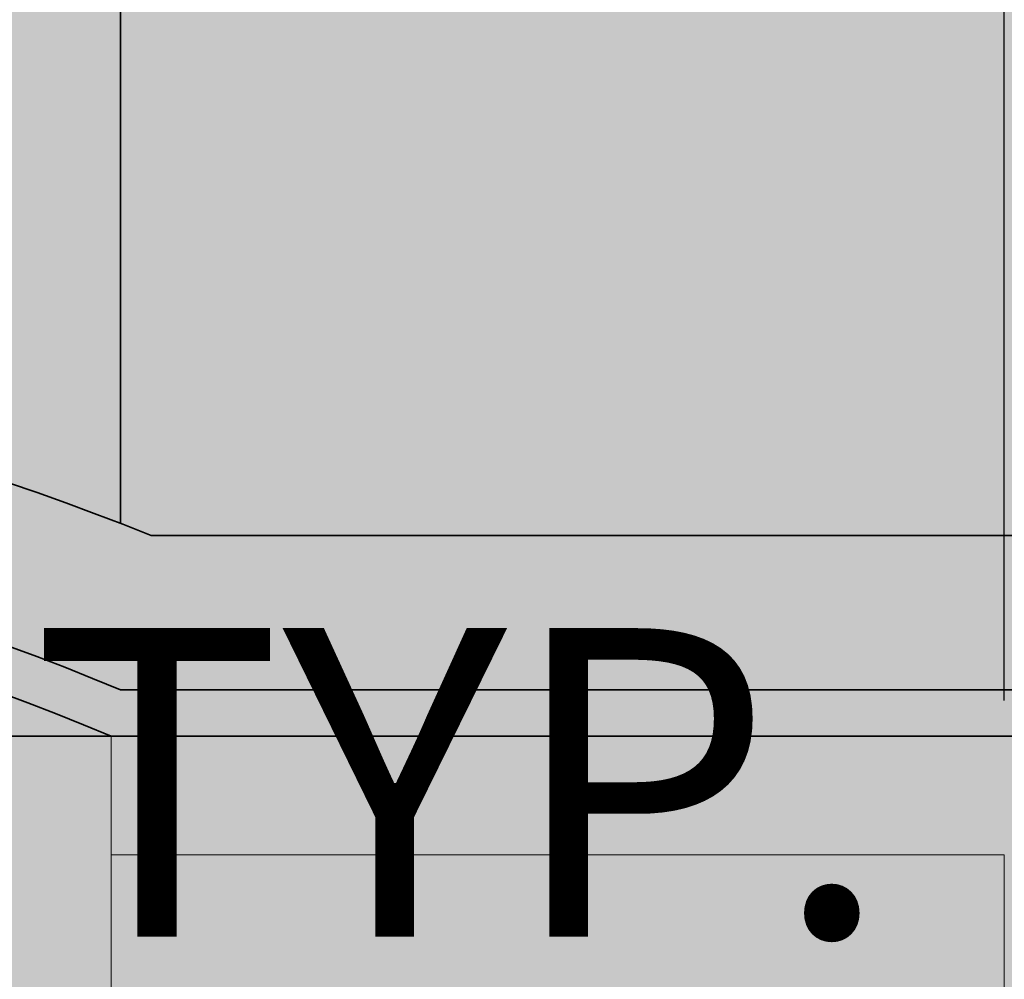
# Model space of a CAD drawing. Units: millimetres. Extents: x 130 to 1021, y 147 to 699.
# Tile 12 of 40: x 481 to 545, y 378 to 440. Entities that reach past the tile are written whole.
import ezdxf

# ---------------------------------------------------------------- set-up
doc = ezdxf.new("R2010")
doc.units = ezdxf.units.MM
doc.header["$MEASUREMENT"] = 0
for name, color, linetype, lineweight in [('A-ANNO-DIMS', 2, 'Continuous', 18), ('A-DOOR', 3, 'Continuous', 25), ('A-ELEV', 7, 'Continuous', 35), ('A-ELEV-PATT', 9, 'Continuous', 13), ('A-GLAZ', 4, 'Continuous', 18)]:
    doc.layers.add(name, color=color, linetype=linetype, lineweight=lineweight)
doc.styles.get("Standard").update_dxf_attribs({"font": 'arial.ttf'})
doc.dimstyles.get("Standard").update_dxf_attribs({"dimtxt": 20, "dimasz": 10, "dimexe": 10, "dimexo": 10, "dimgap": 5, "dimtad": 0, "dimtih": 1, "dimtoh": 1, "dimdec": 0, "dimzin": 0, "dimdsep": 46, "dimtxsty": 'Standard', "dimcen": 5, "dimadec": 0, "dimazin": 0, "dimtfac": 1, "dimtdec": 0, "dimtofl": 0, "dimtmove": 0, "dimatfit": 3, "dimfxl": 1, "dimtolj": 1, "dimtzin": 0, "dimarcsym": 0})

# ---------------------------------------------------------------- blocks, each defined once
blk = doc.blocks.new('*D7')
at = {"layer": 'A-ANNO-DIMS', "color": 0, "lineweight": -2, "transparency": 16777216}
for p, q in [((399.374, 349.447), (413.374, 349.447)), ((423.374, 349.447), (433.374, 349.447)), ((389.374, 344.547), (389.374, 339.447)), ((423.374, 344.547), (423.374, 339.447))]:
    blk.add_line(p, q, dxfattribs=at)
at = {"layer": 'A-ANNO-DIMS', "color": 0, "transparency": 16777216}
for points in [[(399.374, 351.114), (399.374, 347.781), (389.374, 349.447)], [(413.374, 351.114), (413.374, 347.781), (423.374, 349.447)]]:
    blk.add_solid(points, dxfattribs=at)
at = {"layer": 'Defpoints', "color": 0, "transparency": 16777216}
for p in [(389.374, 354.547), (423.374, 354.547), (423.374, 349.447)]:
    blk.add_point(p, dxfattribs=at)
at = {"layer": 'A-ANNO-DIMS', "color": 0, "transparency": 16777216, "insert": (582.037, 349.447), "char_height": 20, "attachment_point": 5}
blk.add_mtext('\\A1;DOOR PANEL 34 TYP.', dxfattribs=at)
blk = doc.blocks.new('*D8')
at = {"layer": 'A-ANNO-DIMS', "color": 0, "lineweight": -2, "transparency": 16777216}
for p, q in [((428.474, 380.947), (428.474, 390.947)), ((428.474, 390.947), (438.474, 390.947)), ((433.374, 370.947), (438.474, 370.947)), ((433.374, 354.547), (438.474, 354.547)), ((428.474, 344.547), (428.474, 334.547))]:
    blk.add_line(p, q, dxfattribs=at)
at = {"layer": 'A-ANNO-DIMS', "color": 0, "transparency": 16777216}
for points in [[(426.807, 380.947), (430.14, 380.947), (428.474, 370.947)], [(426.807, 344.547), (430.14, 344.547), (428.474, 354.547)]]:
    blk.add_solid(points, dxfattribs=at)
at = {"layer": 'Defpoints', "color": 0, "transparency": 16777216}
for p in [(423.374, 370.947), (428.474, 370.947), (423.374, 354.547)]:
    blk.add_point(p, dxfattribs=at)
at = {"layer": 'A-ANNO-DIMS', "color": 0, "transparency": 16777216, "insert": (491.209, 390.947), "char_height": 20, "attachment_point": 5}
blk.add_mtext('\\A1;16 TYP.', dxfattribs=at)
blk = doc.blocks.new('*D11')
at = {"layer": 'A-ANNO-DIMS', "color": 0, "lineweight": -2, "transparency": 16777216}
for p, q in [((737.374, 648.699), (737.374, 149.739)), ((299.374, 566.947), (299.374, 149.739)), ((309.374, 159.739), (490.857, 159.739)), ((727.374, 159.739), (545.891, 159.739))]:
    blk.add_line(p, q, dxfattribs=at)
at = {"layer": 'A-ANNO-DIMS', "color": 0, "transparency": 16777216}
for points in [[(309.374, 161.406), (309.374, 158.073), (299.374, 159.739)], [(727.374, 161.406), (727.374, 158.073), (737.374, 159.739)]]:
    blk.add_solid(points, dxfattribs=at)
at = {"layer": 'Defpoints', "color": 0, "transparency": 16777216}
for p in [(737.374, 658.699), (299.374, 576.947), (737.374, 159.739)]:
    blk.add_point(p, dxfattribs=at)
at = {"layer": 'A-ANNO-DIMS', "color": 0, "transparency": 16777216, "insert": (518.374, 159.739), "char_height": 20, "attachment_point": 5}
blk.add_mtext('\\A1;438', dxfattribs=at)
blk = doc.blocks.new('*D12')
at = {"layer": 'A-ANNO-DIMS', "color": 0, "lineweight": -2, "transparency": 16777216}
for p, q in [((477.374, 661.947), (265.074, 661.947)), ((275.074, 651.947), (275.074, 438.205)), ((275.074, 194.039), (275.074, 407.782)), ((357.163, 184.039), (265.074, 184.039))]:
    blk.add_line(p, q, dxfattribs=at)
at = {"layer": 'A-ANNO-DIMS', "color": 0, "transparency": 16777216}
for points in [[(273.407, 651.947), (276.74, 651.947), (275.074, 661.947)], [(273.407, 194.039), (276.74, 194.039), (275.074, 184.039)]]:
    blk.add_solid(points, dxfattribs=at)
at = {"layer": 'Defpoints', "color": 0, "transparency": 16777216}
for p in [(275.074, 661.947), (487.374, 661.947), (367.163, 184.039)]:
    blk.add_point(p, dxfattribs=at)
at = {"layer": 'A-ANNO-DIMS', "color": 0, "transparency": 16777216, "insert": (275.074, 422.993), "char_height": 20, "attachment_point": 5}
blk.add_mtext('\\A1;477.9', dxfattribs=at)
blk = doc.blocks.new('*D19')
at = {"layer": 'A-ANNO-DIMS', "color": 0, "lineweight": -2, "transparency": 16777216}
for p, q in [((382.374, 388.947), (382.374, 696.247)), ((414.652, 510.881), (414.652, 696.247)), ((392.374, 686.247), (404.652, 686.247)), ((414.652, 686.247), (424.652, 686.247))]:
    blk.add_line(p, q, dxfattribs=at)
at = {"layer": 'A-ANNO-DIMS', "color": 0, "transparency": 16777216}
for points in [[(392.374, 687.914), (392.374, 684.581), (382.374, 686.247)], [(404.652, 687.914), (404.652, 684.581), (414.652, 686.247)]]:
    blk.add_solid(points, dxfattribs=at)
at = {"layer": 'Defpoints', "color": 0, "transparency": 16777216}
for p in [(414.652, 686.247), (414.652, 500.881), (382.374, 378.947)]:
    blk.add_point(p, dxfattribs=at)
at = {"layer": 'A-ANNO-DIMS', "color": 0, "transparency": 16777216, "insert": (463.411, 686.247), "char_height": 20, "attachment_point": 5}
blk.add_mtext('\\A1;32.28', dxfattribs=at)
blk = doc.blocks.new('*D20')
at = {"layer": 'A-ANNO-DIMS', "color": 0, "lineweight": -2, "transparency": 16777216}
for p, q in [((414.652, 510.881), (414.652, 696.247)), ((432.374, 388.947), (432.374, 696.247)), ((404.652, 686.247), (394.652, 686.247)), ((442.374, 686.247), (452.374, 686.247))]:
    blk.add_line(p, q, dxfattribs=at)
at = {"layer": 'A-ANNO-DIMS', "color": 0, "transparency": 16777216}
for points in [[(404.652, 687.914), (404.652, 684.581), (414.652, 686.247)], [(442.374, 687.914), (442.374, 684.581), (432.374, 686.247)]]:
    blk.add_solid(points, dxfattribs=at)
at = {"layer": 'Defpoints', "color": 0, "transparency": 16777216}
for p in [(432.374, 686.247), (414.652, 500.881), (432.374, 378.947)]:
    blk.add_point(p, dxfattribs=at)
at = {"layer": 'A-ANNO-DIMS', "color": 0, "transparency": 16777216, "insert": (490.075, 686.247), "char_height": 20, "attachment_point": 5}
blk.add_mtext('\\A1;17.72', dxfattribs=at)
blk = doc.blocks.new('*D21')
at = {"layer": 'A-ANNO-DIMS', "color": 0, "lineweight": -2, "transparency": 16777216}
for p, q in [((432.374, 388.947), (432.374, 696.247)), ((447.374, 656.947), (447.374, 696.247)), ((422.374, 686.247), (412.374, 686.247)), ((457.374, 686.247), (467.374, 686.247))]:
    blk.add_line(p, q, dxfattribs=at)
at = {"layer": 'A-ANNO-DIMS', "color": 0, "transparency": 16777216}
for points in [[(422.374, 687.914), (422.374, 684.581), (432.374, 686.247)], [(457.374, 687.914), (457.374, 684.581), (447.374, 686.247)]]:
    blk.add_solid(points, dxfattribs=at)
at = {"layer": 'Defpoints', "color": 0, "transparency": 16777216}
for p in [(447.374, 686.247), (447.374, 646.947), (432.374, 378.947)]:
    blk.add_point(p, dxfattribs=at)
at = {"layer": 'A-ANNO-DIMS', "color": 0, "transparency": 16777216, "insert": (485.832, 686.247), "char_height": 20, "attachment_point": 5}
blk.add_mtext('\\A1;15', dxfattribs=at)
blk = doc.blocks.new('*D22')
at = {"layer": 'A-ANNO-DIMS', "color": 0, "lineweight": -2, "transparency": 16777216}
for p, q in [((447.374, 656.947), (447.374, 696.247)), ((466.767, 403.947), (466.767, 696.247)), ((437.374, 686.247), (427.374, 686.247)), ((476.767, 686.247), (486.767, 686.247))]:
    blk.add_line(p, q, dxfattribs=at)
at = {"layer": 'A-ANNO-DIMS', "color": 0, "transparency": 16777216}
for points in [[(437.374, 687.914), (437.374, 684.581), (447.374, 686.247)], [(476.767, 687.914), (476.767, 684.581), (466.767, 686.247)]]:
    blk.add_solid(points, dxfattribs=at)
at = {"layer": 'Defpoints', "color": 0, "transparency": 16777216}
for p in [(466.767, 686.247), (447.374, 646.947), (466.767, 393.947)]:
    blk.add_point(p, dxfattribs=at)
at = {"layer": 'A-ANNO-DIMS', "color": 0, "transparency": 16777216, "insert": (532.34, 686.247), "char_height": 20, "attachment_point": 5}
blk.add_mtext('\\A1;19.393', dxfattribs=at)
blk = doc.blocks.new('*D23')
at = {"layer": 'A-ANNO-DIMS', "color": 0, "lineweight": -2, "transparency": 16777216}
for p, q in [((466.767, 403.947), (466.767, 696.247)), ((475.988, 209.039), (475.988, 696.247)), ((456.767, 686.247), (446.767, 686.247)), ((485.988, 686.247), (495.988, 686.247))]:
    blk.add_line(p, q, dxfattribs=at)
at = {"layer": 'A-ANNO-DIMS', "color": 0, "transparency": 16777216}
for points in [[(456.767, 687.914), (456.767, 684.581), (466.767, 686.247)], [(485.988, 687.914), (485.988, 684.581), (475.988, 686.247)]]:
    blk.add_solid(points, dxfattribs=at)
at = {"layer": 'Defpoints', "color": 0, "transparency": 16777216}
for p in [(475.988, 686.247), (466.767, 393.947), (475.988, 199.039)]:
    blk.add_point(p, dxfattribs=at)
at = {"layer": 'A-ANNO-DIMS', "color": 0, "transparency": 16777216, "insert": (534.631, 686.247), "char_height": 20, "attachment_point": 5}
blk.add_mtext('\\A1;9.222', dxfattribs=at)
blk = doc.blocks.new('*D24')
at = {"layer": 'A-ANNO-DIMS', "color": 0, "lineweight": -2, "transparency": 16777216}
for p, q in [((475.988, 209.039), (475.988, 696.247)), ((487.374, 671.947), (487.374, 696.247)), ((465.988, 686.247), (455.988, 686.247)), ((497.374, 686.247), (507.374, 686.247))]:
    blk.add_line(p, q, dxfattribs=at)
at = {"layer": 'A-ANNO-DIMS', "color": 0, "transparency": 16777216}
for points in [[(465.988, 687.914), (465.988, 684.581), (475.988, 686.247)], [(497.374, 687.914), (497.374, 684.581), (487.374, 686.247)]]:
    blk.add_solid(points, dxfattribs=at)
at = {"layer": 'Defpoints', "color": 0, "transparency": 16777216}
for p in [(487.374, 686.247), (487.374, 661.947), (475.988, 199.039)]:
    blk.add_point(p, dxfattribs=at)
at = {"layer": 'A-ANNO-DIMS', "color": 0, "transparency": 16777216, "insert": (553.022, 686.247), "char_height": 20, "attachment_point": 5}
blk.add_mtext('\\A1;11.385', dxfattribs=at)
blk = doc.blocks.new('*D27')
at = {"layer": 'A-ANNO-DIMS', "color": 0, "lineweight": -2, "transparency": 16777216}
for p, q in [((502.374, 593.947), (502.374, 696.247)), ((544.635, 396.264), (544.635, 696.247)), ((512.374, 686.247), (534.635, 686.247)), ((544.635, 686.247), (554.635, 686.247))]:
    blk.add_line(p, q, dxfattribs=at)
at = {"layer": 'A-ANNO-DIMS', "color": 0, "transparency": 16777216}
for points in [[(512.374, 687.914), (512.374, 684.581), (502.374, 686.247)], [(534.635, 687.914), (534.635, 684.581), (544.635, 686.247)]]:
    blk.add_solid(points, dxfattribs=at)
at = {"layer": 'Defpoints', "color": 0, "transparency": 16777216}
for p in [(544.635, 686.247), (502.374, 583.947), (544.635, 386.264)]:
    blk.add_point(p, dxfattribs=at)
at = {"layer": 'A-ANNO-DIMS', "color": 0, "transparency": 16777216, "insert": (593.776, 686.247), "char_height": 20, "attachment_point": 5}
blk.add_mtext('\\A1;42.26', dxfattribs=at)
blk = doc.blocks.new('*D28')
at = {"layer": 'A-ANNO-DIMS', "color": 0, "lineweight": -2, "transparency": 16777216}
for p, q in [((544.635, 396.264), (544.635, 696.247)), ((552.374, 593.947), (552.374, 696.247)), ((534.635, 686.247), (524.635, 686.247)), ((562.374, 686.247), (572.374, 686.247))]:
    blk.add_line(p, q, dxfattribs=at)
at = {"layer": 'A-ANNO-DIMS', "color": 0, "transparency": 16777216}
for points in [[(534.635, 687.914), (534.635, 684.581), (544.635, 686.247)], [(562.374, 687.914), (562.374, 684.581), (552.374, 686.247)]]:
    blk.add_solid(points, dxfattribs=at)
at = {"layer": 'Defpoints', "color": 0, "transparency": 16777216}
for p in [(552.374, 686.247), (552.374, 583.947), (544.635, 386.264)]:
    blk.add_point(p, dxfattribs=at)
at = {"layer": 'A-ANNO-DIMS', "color": 0, "transparency": 16777216, "insert": (611.057, 686.247), "char_height": 20, "attachment_point": 5}
blk.add_mtext('\\A1;7.738', dxfattribs=at)
blk = doc.blocks.new('*D54')
at = {"layer": 'A-ANNO-DIMS', "color": 0, "lineweight": -2, "transparency": 16777216}
for p, q in [((761.674, 473.947), (761.674, 483.947)), ((497.374, 463.947), (771.674, 463.947)), ((747.374, 403.69), (771.674, 403.69)), ((761.674, 393.69), (761.674, 383.69))]:
    blk.add_line(p, q, dxfattribs=at)
at = {"layer": 'A-ANNO-DIMS', "color": 0, "transparency": 16777216}
for points in [[(760.007, 473.947), (763.34, 473.947), (761.674, 463.947)], [(760.007, 393.69), (763.34, 393.69), (761.674, 403.69)]]:
    blk.add_solid(points, dxfattribs=at)
at = {"layer": 'Defpoints', "color": 0, "transparency": 16777216}
for p in [(487.374, 463.947), (761.674, 463.947), (737.374, 403.69)]:
    blk.add_point(p, dxfattribs=at)
at = {"layer": 'A-ANNO-DIMS', "color": 0, "transparency": 16777216, "insert": (761.674, 433.819), "char_height": 20, "attachment_point": 5}
blk.add_mtext('\\A1;60.26', dxfattribs=at)
blk = doc.blocks.new('*D64')
at = {"layer": 'A-ANNO-DIMS', "color": 0, "lineweight": -2, "transparency": 16777216}
for p, q in [((502.049, 450.926), (502.049, 460.926)), ((497.049, 455.926), (507.049, 455.926)), ((363.96, 263.061), (409.922, 327.255)), ((353.96, 263.061), (363.96, 263.061))]:
    blk.add_line(p, q, dxfattribs=at)
at = {"layer": 'A-ANNO-DIMS', "color": 0, "transparency": 16777216}
blk.add_solid([(408.567, 328.225), (411.277, 326.284), (415.743, 335.385)], dxfattribs=at)
at = {"layer": 'Defpoints', "color": 0, "transparency": 16777216}
for p in [(502.049, 455.926), (415.743, 335.385)]:
    blk.add_point(p, dxfattribs=at)
at = {"layer": 'A-ANNO-DIMS', "color": 0, "transparency": 16777216, "insert": (297.8, 263.061), "char_height": 20, "attachment_point": 5}
blk.add_mtext('\\A1;R148.25', dxfattribs=at)
blk = doc.blocks.new('*D65')
at = {"layer": 'A-ANNO-DIMS', "color": 0, "lineweight": -2, "transparency": 16777216}
for p, q in [((495.463, 509.127), (472.508, 423.108)), ((505.463, 509.127), (495.463, 509.127)), ((427.374, 248.979), (427.374, 258.979)), ((422.374, 253.979), (432.374, 253.979))]:
    blk.add_line(p, q, dxfattribs=at)
at = {"layer": 'A-ANNO-DIMS', "color": 0, "transparency": 16777216}
blk.add_solid([(470.898, 423.538), (474.118, 422.679), (469.93, 413.447)], dxfattribs=at)
at = {"layer": 'Defpoints', "color": 0, "transparency": 16777216}
for p in [(469.93, 413.447), (427.374, 253.979)]:
    blk.add_point(p, dxfattribs=at)
at = {"layer": 'A-ANNO-DIMS', "color": 0, "transparency": 16777216, "insert": (561.623, 509.127), "char_height": 20, "attachment_point": 5}
blk.add_mtext('\\A1;R165.05', dxfattribs=at)
blk = doc.blocks.new('*D67')
at = {"layer": 'A-ANNO-DIMS', "color": 0, "lineweight": -2, "transparency": 16777216}
for p, q in [((479.756, 492.431), (462.144, 412.223)), ((489.756, 492.431), (479.756, 492.431)), ((427.07, 247.496), (427.07, 257.496)), ((422.07, 252.496), (432.07, 252.496))]:
    blk.add_line(p, q, dxfattribs=at)
at = {"layer": 'A-ANNO-DIMS', "color": 0, "transparency": 16777216}
blk.add_solid([(460.516, 412.58), (463.772, 411.865), (459.999, 402.455)], dxfattribs=at)
at = {"layer": 'Defpoints', "color": 0, "transparency": 16777216}
for p in [(459.999, 402.455), (427.07, 252.496)]:
    blk.add_point(p, dxfattribs=at)
at = {"layer": 'A-ANNO-DIMS', "color": 0, "transparency": 16777216, "insert": (545.841, 492.431), "char_height": 20, "attachment_point": 5}
blk.add_mtext('\\A1;R153.53', dxfattribs=at)
blk = doc.blocks.new('*D69')
at = {"layer": 'A-ANNO-DIMS', "color": 0, "lineweight": -2, "transparency": 16777216}
for p, q in [((507.746, 572.261), (483.091, 501.813)), ((517.746, 572.261), (507.746, 572.261)), ((433.191, 354.23), (433.191, 364.23)), ((428.191, 359.23), (438.191, 359.23))]:
    blk.add_line(p, q, dxfattribs=at)
at = {"layer": 'A-ANNO-DIMS', "color": 0, "transparency": 16777216}
blk.add_solid([(481.518, 502.363), (484.664, 501.262), (479.788, 492.374)], dxfattribs=at)
at = {"layer": 'Defpoints', "color": 0, "transparency": 16777216}
for p in [(479.788, 492.374), (433.191, 359.23)]:
    blk.add_point(p, dxfattribs=at)
at = {"layer": 'A-ANNO-DIMS', "color": 0, "transparency": 16777216, "insert": (573.824, 572.261), "char_height": 20, "attachment_point": 5}
blk.add_mtext('\\A1;R141.06', dxfattribs=at)
blk = doc.blocks.new('*D71')
at = {"layer": 'A-ANNO-DIMS', "color": 0, "lineweight": -2, "transparency": 16777216}
for p, q in [((492.108, 581.609), (472.542, 512.666)), ((502.108, 581.609), (492.108, 581.609)), ((432.65, 367.109), (432.65, 377.109)), ((427.65, 372.109), (437.65, 372.109))]:
    blk.add_line(p, q, dxfattribs=at)
at = {"layer": 'A-ANNO-DIMS', "color": 0, "transparency": 16777216}
blk.add_solid([(470.938, 513.121), (474.145, 512.211), (469.812, 503.046)], dxfattribs=at)
at = {"layer": 'Defpoints', "color": 0, "transparency": 16777216}
for p in [(469.812, 503.046), (432.65, 372.109)]:
    blk.add_point(p, dxfattribs=at)
at = {"layer": 'A-ANNO-DIMS', "color": 0, "transparency": 16777216, "insert": (548.493, 581.609), "char_height": 20, "attachment_point": 5}
blk.add_mtext('\\A1;R136.1', dxfattribs=at)
blk = doc.blocks.new('*D72')
at = {"layer": 'A-ANNO-DIMS', "color": 0, "lineweight": -2, "transparency": 16777216}
for p, q in [((460.658, 573.64), (451.279, 503.49)), ((470.658, 573.64), (460.658, 573.64)), ((432.115, 355.142), (432.115, 365.142)), ((427.115, 360.142), (437.115, 360.142))]:
    blk.add_line(p, q, dxfattribs=at)
at = {"layer": 'A-ANNO-DIMS', "color": 0, "transparency": 16777216}
blk.add_solid([(449.628, 503.711), (452.931, 503.27), (449.954, 493.579)], dxfattribs=at)
at = {"layer": 'Defpoints', "color": 0, "transparency": 16777216}
for p in [(449.954, 493.579), (432.115, 360.142)]:
    blk.add_point(p, dxfattribs=at)
at = {"layer": 'A-ANNO-DIMS', "color": 0, "transparency": 16777216, "insert": (526.64, 573.64), "char_height": 20, "attachment_point": 5}
blk.add_mtext('\\A1;R134.62', dxfattribs=at)

msp = doc.modelspace()

# ---------------------------------------------------------------- hatches: boundary and pattern name
at = {"layer": 'A-ELEV-PATT'}
h = msp.add_hatch(color=256, dxfattribs=at)
h.dxf.hatch_style = 1
h.paths.add_polyline_path([(737.3738, 658.6988, 0.0135961), (632.4019, 661.9473), (607.3738, 661.9473), (487.3738, 661.9473), (487.3738, 649.9473), (607.3738, 649.9473), (632.3794, 649.9473, -0.0136841), (737.3738, 646.6784)])
h.paths.add_polyline_path([(732.3738, 643.9599, 0.0130529), (632.3738, 646.9473), (607.3738, 646.9473), (487.3738, 646.9473), (487.3738, 596.9473), (632.3738, 596.9473, -0.0130529), (732.3738, 593.9599)])
h.paths.add_polyline_path([(737.3738, 593.6732, 0.0137063), (632.3738, 596.9473), (487.3738, 596.9473), (487.3738, 586.9473), (632.355, 586.9473, -0.0137808), (737.3738, 583.6559)])
h.paths.add_polyline_path([(447.3738, 646.9473), (307.3738, 646.9473), (302.3738, 646.9473), (302.3738, 634.9473), (447.3738, 634.9473)])
h.paths.add_polyline_path([(447.3738, 631.9473), (307.3738, 631.9473), (307.3738, 586.9473), (447.3738, 586.9473)])
h.paths.add_polyline_path([(447.3738, 586.9473), (307.3738, 586.9473), (302.3738, 586.9473), (302.3738, 576.9473), (447.3738, 576.9473)])
h.paths.add_polyline_path([(447.3738, 573.9473), (367.3738, 573.9473), (367.3738, 539.9473), (447.3738, 539.9473)])
h.paths.add_polyline_path([(447.3738, 537.9473), (367.3738, 537.9473), (367.3738, 507.9473), (400.392, 507.4253, -0.001728), (401.3281, 507.6451, -0.5220025), (425.6117, 511.0391, -0.0391849), (447.3738, 510.4359), (447.3738, 510.7883)])
h.paths.add_polyline_path([(394.7238, 505.9473), (367.3738, 505.9473), (367.3738, 476.9473, -0.0146512), (375.8501, 480.2159), (376.1506, 499.2266, -0.0355419)])
h.paths.add_polyline_path([(632.3738, 583.9473), (552.3738, 583.9473), (552.3738, 550.9473), (632.3738, 550.9473)])
h.paths.add_polyline_path([(632.3738, 548.9473), (552.3738, 548.9473), (552.3738, 515.9473), (632.3738, 515.9473)])
h.paths.add_polyline_path([(632.3738, 513.9473), (552.3738, 513.9473), (552.3738, 476.9473), (632.3738, 476.9473)])
h.paths.add_polyline_path([(737.3738, 473.6903, 0.0136326), (632.3926, 476.9473), (552.3738, 476.9473), (487.3738, 476.9473), (487.3738, 466.9473), (632.3738, 466.9473, -0.0137063), (737.3738, 463.6732)])
h.paths.add_polyline_path([(732.3738, 460.9552, 0.0130741), (632.3681, 463.9473), (487.3738, 463.9473), (487.3738, 407.735, -0.0032286), (489.3544, 406.9473), (632.3926, 406.9473, -0.0129826), (732.3738, 403.9755)])
h.paths.add_polyline_path([(487.3738, 463.9473, 0.20133), (367.3738, 463.9473), (367.3738, 407.735, -0.1882031), (487.3738, 407.735)])
h.paths.add_polyline_path([(367.3738, 476.9473), (367.3738, 466.9473, -0.2013309), (487.3738, 466.9473), (487.3738, 476.9473, 0.20133)])
h.paths.add_polyline_path([(367.3738, 463.9473), (307.3738, 463.9473), (307.3738, 401.9473), (357.9413, 401.9473), (367.3738, 407.735)])
h.paths.add_polyline_path([(367.3738, 476.9473), (302.3738, 476.9473), (302.3738, 466.9473), (367.3738, 466.9473)])
h.paths.add_polyline_path([(632.8184, 366.9453), (552.3738, 366.9453), (552.3738, 393.9473), (632.8184, 393.9473)])
h.paths.add_polyline_path([(632.8184, 357.2114), (632.8184, 363.9453), (552.3738, 363.9453), (552.3738, 357.2114), (552.3738, 336.9453), (632.8184, 336.9453)])
h.paths.add_polyline_path([(632.8184, 333.9453), (552.3738, 333.9453), (552.3738, 306.9453), (632.8184, 306.9453)])
h.paths.add_polyline_path([(632.8184, 303.9453), (552.3738, 303.9453), (552.3738, 273.9473), (632.355, 273.9473, 0.0000608), (632.8184, 273.9491)])
h.paths.add_polyline_path([(737.3738, 403.6903, 0.0136326), (632.3926, 406.9473), (489.3544, 406.9473, 0.1915481), (367.3738, 407.735), (367.3738, 396.9473, -0.2013309), (487.3738, 396.9473), (632.3738, 396.9473, -0.0137063), (737.3738, 393.6732)])
h.paths.add_polyline_path([(357.9413, 401.9473), (307.3738, 401.9473), (307.3738, 391.9473), (357.9413, 391.9473)])
h.paths.add_polyline_path([(357.9413, 357.2114), (357.9413, 388.9473), (307.3738, 388.9473), (307.3738, 357.2114), (307.3738, 273.9473), (357.9413, 273.9473)])
h.paths.add_polyline_path([(732.3738, 263.93, -0.0130317), (632.3794, 260.9473), (466.7667, 260.9473), (466.7667, 240.9473), (469.8406, 236.978), (469.8406, 221.978), (472.9145, 218.0087), (472.9145, 213.9473), (607.3738, 213.9473), (732.3738, 213.9473)])
h.paths.add_polyline_path([(732.3738, 290.889), (722.479, 290.889), (722.479, 301.889), (732.3738, 301.889), (732.3738, 305.889), (722.479, 305.889), (722.479, 316.889), (732.3738, 316.889), (732.3738, 320.889), (722.479, 320.889), (722.479, 331.889), (732.3738, 331.889), (732.3738, 335.889), (722.479, 335.889), (722.479, 346.889), (732.3738, 346.889), (732.3738, 350.889), (722.479, 350.889), (722.479, 361.889), (732.3738, 361.889), (732.3738, 365.889), (722.479, 365.889), (722.479, 376.889), (732.3738, 376.889), (732.3738, 380.889), (722.479, 380.889), (722.479, 391.4848, 0.0005233), (718.479, 391.6843), (718.479, 380.889), (707.479, 380.889), (707.479, 392.1896, 0.0005231), (703.479, 392.3576), (703.479, 380.889), (692.479, 380.889), (692.479, 392.7765, 0.0005229), (688.479, 392.9131), (688.479, 380.889), (677.479, 380.889), (677.479, 393.2456, 0.0005228), (673.479, 393.3508), (673.479, 380.889), (662.479, 380.889), (662.479, 393.597, 0.0005227), (658.479, 393.6709), (658.479, 380.889), (647.479, 380.889), (647.479, 393.8308, 0.0005226), (643.479, 393.8732), (643.479, 380.889), (632.8184, 380.889), (632.8184, 376.889), (643.479, 376.889), (643.479, 365.889), (632.8184, 365.889), (632.8184, 361.889), (643.479, 361.889), (643.479, 350.889), (632.8184, 350.889), (632.8184, 346.889), (643.479, 346.889), (643.479, 335.889), (632.8184, 335.889), (632.8184, 331.889), (643.479, 331.889), (643.479, 320.889), (632.8184, 320.889), (632.8184, 316.889), (643.479, 316.889), (643.479, 305.889), (632.8184, 305.889), (632.8184, 301.889), (643.479, 301.889), (643.479, 290.889), (632.8184, 290.889), (632.8184, 286.889), (643.479, 286.889), (643.479, 274.0217, 0.0005246), (647.479, 274.0643), (647.479, 286.889), (658.479, 286.889), (658.479, 274.2248, 0.0005246), (662.479, 274.2989), (662.479, 286.889), (673.479, 286.889), (673.479, 274.546, 0.0005247), (677.479, 274.6516), (677.479, 286.889), (688.479, 286.889), (688.479, 274.9853, 0.0005248), (692.479, 275.1224), (692.479, 286.889), (703.479, 286.889), (703.479, 275.5429, 0.000525), (707.479, 275.7115), (707.479, 286.889), (718.479, 286.889), (718.479, 276.2187, 0.0005252), (722.479, 276.4189), (722.479, 286.889), (732.3738, 286.889)])
h.paths.add_polyline_path([(718.479, 290.889), (707.479, 290.889), (707.479, 301.889), (718.479, 301.889)], flags=16)
h.paths.add_polyline_path([(703.479, 290.889), (692.479, 290.889), (692.479, 301.889), (703.479, 301.889)], flags=16)
h.paths.add_polyline_path([(718.479, 305.889), (707.479, 305.889), (707.479, 316.889), (718.479, 316.889)], flags=16)
h.paths.add_polyline_path([(703.479, 305.889), (692.479, 305.889), (692.479, 316.889), (703.479, 316.889)], flags=16)
h.paths.add_polyline_path([(688.479, 290.889), (677.479, 290.889), (677.479, 301.889), (688.479, 301.889)], flags=16)
h.paths.add_polyline_path([(718.479, 320.889), (707.479, 320.889), (707.479, 331.889), (718.479, 331.889)], flags=16)
h.paths.add_polyline_path([(688.479, 305.889), (677.479, 305.889), (677.479, 316.889), (688.479, 316.889)], flags=16)
h.paths.add_polyline_path([(703.479, 320.889), (692.479, 320.889), (692.479, 331.889), (703.479, 331.889)], flags=16)
h.paths.add_polyline_path([(688.479, 320.889), (677.479, 320.889), (677.479, 331.889), (688.479, 331.889)], flags=16)
h.paths.add_polyline_path([(673.479, 290.889), (662.479, 290.889), (662.479, 301.889), (673.479, 301.889)], flags=16)
h.paths.add_polyline_path([(718.479, 335.889), (707.479, 335.889), (707.479, 346.889), (718.479, 346.889)], flags=16)
h.paths.add_polyline_path([(673.479, 305.889), (662.479, 305.889), (662.479, 316.889), (673.479, 316.889)], flags=16)
h.paths.add_polyline_path([(703.479, 335.889), (692.479, 335.889), (692.479, 346.889), (703.479, 346.889)], flags=16)
h.paths.add_polyline_path([(673.479, 320.889), (662.479, 320.889), (662.479, 331.889), (673.479, 331.889)], flags=16)
h.paths.add_polyline_path([(688.479, 335.889), (677.479, 335.889), (677.479, 346.889), (688.479, 346.889)], flags=16)
h.paths.add_polyline_path([(658.479, 290.889), (647.479, 290.889), (647.479, 301.889), (658.479, 301.889)], flags=16)
h.paths.add_polyline_path([(718.479, 350.889), (707.479, 350.889), (707.479, 361.889), (718.479, 361.889)], flags=16)
h.paths.add_polyline_path([(658.479, 305.889), (647.479, 305.889), (647.479, 316.889), (658.479, 316.889)], flags=16)
h.paths.add_polyline_path([(703.479, 350.889), (692.479, 350.889), (692.479, 361.889), (703.479, 361.889)], flags=16)
h.paths.add_polyline_path([(673.479, 335.889), (662.479, 335.889), (662.479, 346.889), (673.479, 346.889)], flags=16)
h.paths.add_polyline_path([(658.479, 320.889), (647.479, 320.889), (647.479, 331.889), (658.479, 331.889)], flags=16)
h.paths.add_polyline_path([(688.479, 350.889), (677.479, 350.889), (677.479, 361.889), (688.479, 361.889)], flags=16)
h.paths.add_polyline_path([(718.479, 365.889), (707.479, 365.889), (707.479, 376.889), (718.479, 376.889)], flags=16)
h.paths.add_polyline_path([(658.479, 335.889), (647.479, 335.889), (647.479, 346.889), (658.479, 346.889)], flags=16)
h.paths.add_polyline_path([(673.479, 350.889), (662.479, 350.889), (662.479, 361.889), (673.479, 361.889)], flags=16)
h.paths.add_polyline_path([(703.479, 365.889), (692.479, 365.889), (692.479, 376.889), (703.479, 376.889)], flags=16)
h.paths.add_polyline_path([(688.479, 365.889), (677.479, 365.889), (677.479, 376.889), (688.479, 376.889)], flags=16)
h.paths.add_polyline_path([(658.479, 350.889), (647.479, 350.889), (647.479, 361.889), (658.479, 361.889)], flags=16)
h.paths.add_polyline_path([(673.479, 365.889), (662.479, 365.889), (662.479, 376.889), (673.479, 376.889)], flags=16)
h.paths.add_polyline_path([(658.479, 365.889), (647.479, 365.889), (647.479, 376.889), (658.479, 376.889)], flags=16)
h.paths.add_polyline_path([(732.3738, 503.9786), (722.3392, 503.9786), (722.3392, 514.9786), (732.3738, 514.9786), (732.3738, 518.9786), (722.3392, 518.9786), (722.3392, 529.9786), (732.3738, 529.9786), (732.3738, 533.9786), (722.3392, 533.9786), (722.3392, 544.9786), (732.3738, 544.9786), (732.3738, 546.9473), (732.3738, 548.9786), (722.3392, 548.9786), (722.3392, 559.9786), (732.3738, 559.9786), (732.3738, 563.9786), (722.3392, 563.9786), (722.3392, 574.9786), (732.3738, 574.9786), (732.3738, 578.9786), (722.3392, 578.9786), (722.3392, 581.4789, 0.000526), (718.3392, 581.6791), (718.3392, 578.9786), (707.3392, 578.9786), (707.3392, 582.1863, 0.0005258), (703.3392, 582.355), (703.3392, 578.9786), (692.3392, 578.9786), (692.3392, 582.7752, 0.0005257), (688.3392, 582.9123), (688.3392, 578.9786), (677.3392, 578.9786), (677.3392, 583.2457, 0.0005255), (673.3392, 583.3512), (673.3392, 578.9786), (662.3392, 578.9786), (662.3392, 583.5978, 0.0005254), (658.3392, 583.6718), (658.3392, 578.9786), (647.3392, 578.9786), (647.3392, 583.8317, 0.0005254), (643.3392, 583.8741), (643.3392, 578.9786), (632.3738, 578.9786), (632.3738, 574.9786), (643.3392, 574.9786), (643.3392, 563.9786), (632.3738, 563.9786), (632.3738, 559.9786), (643.3392, 559.9786), (643.3392, 548.9786), (632.3738, 548.9786), (632.3738, 544.9786), (643.3392, 544.9786), (643.3392, 533.9786), (632.3738, 533.9786), (632.3738, 529.9786), (643.3392, 529.9786), (643.3392, 518.9786), (632.3738, 518.9786), (632.3738, 515.9473), (632.3738, 514.9786), (643.3392, 514.9786), (643.3392, 503.9786), (632.3738, 503.9786), (632.3738, 499.9786), (643.3392, 499.9786), (643.3392, 488.9786), (632.3738, 488.9786), (632.3738, 484.9786), (643.3392, 484.9786), (643.3392, 476.8751, -0.0005191), (647.3392, 476.8332), (647.3392, 484.9786), (658.3392, 484.9786), (658.3392, 476.6752, -0.0005192), (662.3392, 476.6022), (662.3392, 484.9786), (673.3392, 484.9786), (673.3392, 476.3585, -0.0005193), (677.3392, 476.2543), (677.3392, 484.9786), (688.3392, 484.9786), (688.3392, 475.9248, -0.0005194), (692.3392, 475.7894), (692.3392, 484.9786), (703.3392, 484.9786), (703.3392, 475.3741, -0.0005195), (707.3392, 475.2075), (707.3392, 484.9786), (718.3392, 484.9786), (718.3392, 474.7064, -0.0005197), (722.3392, 474.5086), (722.3392, 484.9786), (732.3738, 484.9786), (732.3738, 488.9786), (722.3392, 488.9786), (722.3392, 499.9786), (732.3738, 499.9786)])
h.paths.add_polyline_path([(718.3392, 503.9786), (707.3392, 503.9786), (707.3392, 514.9786), (718.3392, 514.9786)], flags=16)
h.paths.add_polyline_path([(718.3392, 499.9786), (718.3392, 488.9786), (707.3392, 488.9786), (707.3392, 499.9786)], flags=16)
h.paths.add_polyline_path([(718.3392, 518.9786), (707.3392, 518.9786), (707.3392, 529.9786), (718.3392, 529.9786)], flags=16)
h.paths.add_polyline_path([(703.3392, 503.9786), (692.3392, 503.9786), (692.3392, 514.9786), (703.3392, 514.9786)], flags=16)
h.paths.add_polyline_path([(703.3392, 499.9786), (703.3392, 488.9786), (692.3392, 488.9786), (692.3392, 499.9786)], flags=16)
h.paths.add_polyline_path([(703.3392, 518.9786), (692.3392, 518.9786), (692.3392, 529.9786), (703.3392, 529.9786)], flags=16)
h.paths.add_polyline_path([(718.3392, 533.9786), (707.3392, 533.9786), (707.3392, 544.9786), (718.3392, 544.9786)], flags=16)
h.paths.add_polyline_path([(688.3392, 503.9786), (677.3392, 503.9786), (677.3392, 514.9786), (688.3392, 514.9786)], flags=16)
h.paths.add_polyline_path([(688.3392, 499.9786), (688.3392, 488.9786), (677.3392, 488.9786), (677.3392, 499.9786)], flags=16)
h.paths.add_polyline_path([(703.3392, 533.9786), (692.3392, 533.9786), (692.3392, 544.9786), (703.3392, 544.9786)], flags=16)
h.paths.add_polyline_path([(688.3392, 518.9786), (677.3392, 518.9786), (677.3392, 529.9786), (688.3392, 529.9786)], flags=16)
h.paths.add_polyline_path([(688.3392, 533.9786), (677.3392, 533.9786), (677.3392, 544.9786), (688.3392, 544.9786)], flags=16)
h.paths.add_polyline_path([(718.3392, 548.9786), (707.3392, 548.9786), (707.3392, 559.9786), (718.3392, 559.9786)], flags=16)
h.paths.add_polyline_path([(673.3392, 503.9786), (662.3392, 503.9786), (662.3392, 514.9786), (673.3392, 514.9786)], flags=16)
h.paths.add_polyline_path([(673.3392, 499.9786), (673.3392, 488.9786), (662.3392, 488.9786), (662.3392, 499.9786)], flags=16)
h.paths.add_polyline_path([(703.3392, 548.9786), (692.3392, 548.9786), (692.3392, 559.9786), (703.3392, 559.9786)], flags=16)
h.paths.add_polyline_path([(673.3392, 518.9786), (662.3392, 518.9786), (662.3392, 529.9786), (673.3392, 529.9786)], flags=16)
h.paths.add_polyline_path([(688.3392, 548.9786), (677.3392, 548.9786), (677.3392, 559.9786), (688.3392, 559.9786)], flags=16)
h.paths.add_polyline_path([(673.3392, 533.9786), (662.3392, 533.9786), (662.3392, 544.9786), (673.3392, 544.9786)], flags=16)
h.paths.add_polyline_path([(718.3392, 563.9786), (707.3392, 563.9786), (707.3392, 574.9786), (718.3392, 574.9786)], flags=16)
h.paths.add_polyline_path([(658.3392, 503.9786), (647.3392, 503.9786), (647.3392, 514.9786), (658.3392, 514.9786)], flags=16)
h.paths.add_polyline_path([(658.3392, 499.9786), (658.3392, 488.9786), (647.3392, 488.9786), (647.3392, 499.9786)], flags=16)
h.paths.add_polyline_path([(703.3392, 563.9786), (692.3392, 563.9786), (692.3392, 574.9786), (703.3392, 574.9786)], flags=16)
h.paths.add_polyline_path([(658.3392, 518.9786), (647.3392, 518.9786), (647.3392, 529.9786), (658.3392, 529.9786)], flags=16)
h.paths.add_polyline_path([(673.3392, 548.9786), (662.3392, 548.9786), (662.3392, 559.9786), (673.3392, 559.9786)], flags=16)
h.paths.add_polyline_path([(688.3392, 563.9786), (677.3392, 563.9786), (677.3392, 574.9786), (688.3392, 574.9786)], flags=16)
h.paths.add_polyline_path([(658.3392, 533.9786), (647.3392, 533.9786), (647.3392, 544.9786), (658.3392, 544.9786)], flags=16)
h.paths.add_polyline_path([(673.3392, 563.9786), (662.3392, 563.9786), (662.3392, 574.9786), (673.3392, 574.9786)], flags=16)
h.paths.add_polyline_path([(658.3392, 548.9786), (647.3392, 548.9786), (647.3392, 559.9786), (658.3392, 559.9786)], flags=16)
h.paths.add_polyline_path([(658.3392, 563.9786), (647.3392, 563.9786), (647.3392, 574.9786), (658.3392, 574.9786)], flags=16)
h = msp.add_hatch(color=256, dxfattribs=at)
h.dxf.hatch_style = 1
h.paths.add_polyline_path([(447.3738, 576.9473), (302.3738, 576.9473), (302.3738, 573.9473), (447.3738, 573.9473)])
h.paths.add_polyline_path([(487.3738, 583.9473), (487.3738, 586.9473), (447.3738, 576.9473), (447.3738, 573.9473)])
h.paths.add_polyline_path([(632.355, 586.9473), (487.3738, 586.9473), (487.3738, 583.9473), (632.3738, 583.9473), (632.3738, 583.9472, -0.0138), (737.3738, 580.6507), (737.3738, 583.6559, 0.0137808)])
h.paths.add_polyline_path([(367.3738, 466.9473), (302.3738, 466.9473), (302.3738, 463.9473), (367.3738, 463.9473)])
h.paths.add_polyline_path([(487.3738, 463.9473), (487.3738, 466.9473, 0.2013309), (367.3738, 466.9473), (367.3738, 463.9473, -0.20133)])
h.paths.add_polyline_path([(632.3738, 466.9473), (487.3738, 466.9473), (487.3738, 463.9473), (632.3681, 463.9473, -0.0137285), (737.3738, 460.6681), (737.3738, 463.6732, 0.0137063)])
h.paths.add_polyline_path([(632.3738, 396.9473), (487.3738, 396.9473, 0.2013309), (367.3738, 396.9473), (367.3738, 393.9473, -0.2023717), (486.7667, 393.9473), (632.3681, 393.9473, -0.0137285), (737.3738, 390.6681), (737.3738, 393.6732, 0.0137063)])
h.paths.add_polyline_path([(357.9413, 391.9473), (307.3738, 391.9473), (307.3738, 388.9473), (357.9413, 388.9473)])
h.paths.add_polyline_path([(367.3738, 393.9473), (367.3738, 396.9473), (357.9413, 391.924), (357.9413, 388.9473), (358.058, 388.9473)])
h.paths.add_polyline_path([(737.3738, 264.2162), (737.3738, 267.2214, -0.0137063), (632.3738, 263.9473), (463.7667, 263.9473), (466.7667, 260.9473), (632.3794, 260.9473, 0.0136841)])
h.paths.add_polyline_path([(463.7667, 263.9473), (447.3738, 263.9473), (450.3738, 260.9473), (466.7667, 260.9473)])
h.paths.add_polyline_path([(447.3738, 263.9473), (432.3738, 263.9473), (432.3738, 260.9473), (450.3738, 260.9473)])
h.paths.add_polyline_path([(382.3738, 263.9473), (357.9413, 263.9473), (357.9413, 260.9473), (382.3738, 260.9473)])
h.paths.add_polyline_path([(357.9413, 263.9473), (307.3738, 263.9473), (307.3738, 260.9473), (357.9413, 260.9473)])
h = msp.add_hatch(color=256, dxfattribs=at)
h.paths.add_polyline_path([(327.3738, 569.884), (327.3738, 573.9473), (307.3738, 573.9473), (307.3738, 476.9473), (327.3738, 476.9473), (327.3738, 480.95)])
h.paths.add_polyline_path([(486.7667, 386.2639), (486.7667, 393.9473), (466.7667, 393.9473), (466.7667, 357.2114), (466.7667, 311.9335, 0.0342703), (486.7667, 308.4637)])
h.paths.add_polyline_path([(486.7667, 308.4637, -0.0342703), (466.7667, 311.9335), (466.7667, 273.9473), (486.7667, 273.9473)])
h.paths.add_polyline_path([(389.3738, 351.5473), (396.7693, 351.5473, -0.007027), (393.8774, 354.5473), (389.3738, 354.5473), (389.3738, 359.5775, -0.0190302), (382.3738, 368.424), (382.3738, 249.5473), (432.3738, 249.5473), (432.3738, 325.067, -0.0057673), (429.3738, 326.709), (429.3738, 257.5473), (426.3738, 257.5473), (426.3738, 328.4428, -0.0059254), (423.3738, 330.272), (423.3738, 315.7473), (389.3738, 315.7473), (389.3738, 332.1473), (420.4552, 332.1473, -0.008951), (416.0768, 335.1473), (389.3738, 335.1473)])
h.paths.add_polyline_path([(389.3738, 312.7473), (423.3738, 312.7473), (423.3738, 296.3473), (389.3738, 296.3473)], flags=16)
h.paths.add_polyline_path([(389.3738, 293.3473), (423.3738, 293.3473), (423.3738, 276.9473), (389.3738, 276.9473)], flags=16)
h.paths.add_polyline_path([(389.3738, 273.9473), (423.3738, 273.9473), (423.3738, 257.5473), (389.3738, 257.5473)], flags=16)
h.paths.add_polyline_path([(432.3738, 378.9473), (382.3738, 378.9473), (382.3738, 368.424, 0.0190302), (389.3738, 359.5775), (389.3738, 370.9473), (423.3738, 370.9473), (423.3738, 354.5473), (393.8774, 354.5473, 0.007027), (396.7693, 351.5473), (423.3738, 351.5473), (423.3738, 335.1473), (416.0768, 335.1473, 0.008951), (420.4552, 332.1473), (423.3738, 332.1473), (423.3738, 330.272, 0.0059254), (426.3738, 328.4428), (426.3738, 370.9473), (429.3738, 370.9473), (429.3738, 326.709, 0.0057673), (432.3738, 325.067)])
h.paths.add_polyline_path([(466.7667, 357.2114), (466.7667, 393.9473), (447.3738, 393.9473), (447.3738, 357.2114), (447.3738, 318.1243, 0.0063261), (450.8779, 316.785), (450.8779, 331.5915), (463.5608, 331.5915), (463.5608, 312.7571, 0.005582), (466.7667, 311.9335)])
h.paths.add_polyline_path([(450.8779, 334.5915), (450.8779, 360.0915), (463.5608, 360.0915), (463.5608, 334.5915)], flags=16)
h.paths.add_polyline_path([(450.8779, 363.0915), (450.8779, 388.6449), (463.5608, 388.6449), (463.5608, 363.0915)], flags=16)
h.paths.add_polyline_path([(466.7667, 311.9335, -0.005582), (463.5608, 312.7571), (463.5608, 306.0915), (450.8779, 306.0915), (450.8779, 316.785, -0.0063261), (447.3738, 318.1243), (447.3738, 273.9473), (466.7667, 273.9473)])
h.paths.add_polyline_path([(450.8779, 303.0915), (463.5608, 303.0915), (463.5608, 277.5915), (450.8779, 277.5915)], flags=16)
h.paths.add_polyline_path([(552.3738, 357.2114), (552.3738, 393.9473), (486.7667, 393.9473), (486.7667, 386.2639), (544.6354, 386.2639), (544.6354, 280.6619), (486.7667, 280.6619), (486.7667, 273.9473), (552.3738, 273.9473)])
h.paths.add_polyline_path([(487.3738, 583.9473), (472.3738, 580.1973), (472.3738, 507.0765), (472.3738, 505.4251, -0.0056452), (475.3738, 504.4942), (475.3738, 506.3543), (475.3738, 511.9473), (484.3738, 511.9473), (484.3738, 503.8134), (484.3738, 501.2439, -0.0058357), (487.3738, 500.0015)])
h.paths.add_polyline_path([(484.3738, 578.0434), (484.3738, 548.9473), (475.3738, 548.9473), (475.3738, 575.7934)], flags=16)
h.paths.add_polyline_path([(484.3738, 546.9473), (484.3738, 513.9473), (475.3738, 513.9473), (475.3738, 518.7148), (475.3738, 546.9473)], flags=16)
h = msp.add_hatch(color=256, dxfattribs=at)
h.dxf.hatch_style = 1
h.paths.add_polyline_path([(363.922, 569.884), (327.3738, 569.884), (327.3738, 557.9168), (363.922, 557.9168)])
h.paths.add_polyline_path([(547.7773, 577.3739), (502.3738, 577.3739), (502.3738, 566.2111), (547.7773, 566.2111)])
h.paths.add_polyline_path([(544.6354, 386.2639), (486.7667, 386.2639), (486.7667, 377.43), (544.6354, 377.43)])
h.paths.add_polyline_path([(496.0546, 377.43), (486.7667, 377.43), (486.7667, 370.4028)])
h.paths.add_polyline_path([(447.3738, 393.9473), (367.3738, 393.9473, 0.0500478), (382.3738, 368.424), (382.3738, 378.9473), (432.3738, 378.9473), (432.3738, 325.067, 0.0278945), (447.3738, 318.1243), (447.3738, 357.2114)])
h.paths.add_polyline_path([(463.5608, 388.6449), (450.8779, 388.6449), (450.8779, 363.0915), (463.5608, 363.0915)])
h.paths.add_polyline_path([(463.5608, 360.0915), (450.8779, 360.0915), (450.8779, 334.5915), (463.5608, 334.5915)])
h.paths.add_polyline_path([(463.5608, 331.5915), (450.8779, 331.5915), (450.8779, 316.785, 0.0224513), (463.5608, 312.7571)])
msp.add_hatch(color=256, dxfattribs=at).paths.add_polyline_path([(367.3738, 393.9473), (486.7667, 393.9473, 0.2023717)])

# ---------------------------------------------------------------- linework, layer by layer
at = {"layer": 'A-DOOR'}
msp.add_arc((502.0489, 455.9263), 148.2524, 204.712441, 264.083334, dxfattribs=at)
at = {"layer": 'A-ELEV'}
for p, q in [((487.3738, 407.735), (487.3738, 476.9473)), ((632.3738, 406.9473), (489.3544, 406.9473)), ((632.3738, 396.9473), (487.3738, 396.9473)), ((632.3738, 393.9473), (367.3738, 393.9473))]:
    msp.add_line(p, q, dxfattribs=at)
for centre, radius, start, end in [((427.3738, 253.9788), 165.0484, 67.942927, 111.31713), ((427.3738, 253.9788), 155.0484, 67.233534, 112.766466), ((427.0702, 252.4956), 153.5326, 67.118929, 112.881071)]:
    msp.add_arc(centre, radius, start, end, dxfattribs=at)
at = {"layer": 'A-GLAZ'}
msp.add_line((486.7667, 393.9473), (486.7667, 357.2114), dxfattribs=at)
msp.add_lwpolyline([(544.6354, 386.2639), (486.7667, 386.2639), (486.7667, 280.6619), (544.6354, 280.6619)], close=True, dxfattribs=at)

# ---------------------------------------------------------------- dimensions: what is measured, and where the dimension line sits
at = {"layer": 'A-ANNO-DIMS'}
for base, p1, p2, override, picture, middle in [((414.6525, 686.2473), (382.3738, 378.9473), (414.6525, 500.8811), {"dimdec": 2, "dimlfac": 1, "dimrnd": 0, "dimzin": 0, "dimdsep": 46, "dimlunit": 2}, '*D19', (463.411, 686.2473)), ((432.3738, 686.2473), (414.6525, 500.8811), (432.3738, 378.9473), {"dimdec": 2, "dimlfac": 1, "dimrnd": 0, "dimzin": 0, "dimdsep": 46, "dimlunit": 2}, '*D20', (490.075, 686.2473)), ((447.3738, 686.2473), (432.3738, 378.9473), (447.3738, 646.9473), {"dimdec": 0, "dimlfac": 1, "dimrnd": 0, "dimzin": 0, "dimdsep": 46, "dimlunit": 2}, '*D21', (485.8322, 686.2473)), ((466.7667, 686.2473), (447.3738, 646.9473), (466.7667, 393.9473), {"dimdec": 3, "dimlfac": 1, "dimrnd": 0, "dimzin": 0, "dimdsep": 46, "dimlunit": 2}, '*D22', (532.3397, 686.2473)), ((475.9885, 686.2473), (466.7667, 393.9473), (475.9885, 199.0395), {"dimdec": 3, "dimlfac": 1, "dimrnd": 0, "dimzin": 0, "dimdsep": 46, "dimlunit": 2}, '*D23', (534.631, 686.2473)), ((487.3738, 686.2473), (475.9885, 199.0395), (487.3738, 661.9473), {"dimdec": 3, "dimlfac": 1, "dimrnd": 0, "dimzin": 0, "dimdsep": 46, "dimlunit": 2}, '*D24', (553.0218, 686.2473)), ((544.6354, 686.2473), (502.3738, 583.9473), (544.6354, 386.2639), {"dimdec": 2, "dimlfac": 1, "dimrnd": 0, "dimzin": 0, "dimdsep": 46, "dimlunit": 2}, '*D27', (593.776, 686.2473)), ((552.3738, 686.2473), (544.6354, 386.2639), (552.3738, 583.9473), {"dimdec": 3, "dimlfac": 1, "dimrnd": 0, "dimzin": 0, "dimdsep": 46, "dimlunit": 2}, '*D28', (611.0573, 686.2473)), ((737.3738, 159.7395), (299.3738, 576.9473), (737.3738, 658.6988), {"dimdec": 0, "dimlfac": 1, "dimrnd": 0, "dimzin": 0, "dimdsep": 46, "dimlunit": 2}, '*D11', (518.3738, 159.7395))]:
    dim = msp.add_linear_dim(base=base, p1=p1, p2=p2, dimstyle='Standard', override=override, dxfattribs=at)
    dim.commit()
    dim.dimension.update_dxf_attribs({"geometry": picture, "text_midpoint": middle})
for base, p1, p2, override, picture, middle in [((275.0738, 661.9473), (367.163, 184.0395), (487.3738, 661.9473), {"dimdec": 1, "dimlfac": 1, "dimrnd": 0, "dimzin": 0, "dimdsep": 46, "dimlunit": 2}, '*D12', (275.0738, 422.9934)), ((761.6738, 463.9473), (737.3738, 403.6903), (487.3738, 463.9473), {"dimdec": 2, "dimlfac": 1, "dimrnd": 0, "dimzin": 0, "dimdsep": 46, "dimlunit": 2}, '*D54', (761.6738, 433.8188))]:
    dim = msp.add_linear_dim(base=base, p1=p1, p2=p2, angle=90, dimstyle='Standard', override=override, dxfattribs=at)
    dim.commit()
    dim.dimension.update_dxf_attribs({"geometry": picture, "text_midpoint": middle})
for center, mpoint, override, picture, middle in [((432.6505, 372.1087), (469.8116, 503.0461), {"dimdec": 1, "dimlfac": 1, "dimrnd": 0, "dimzin": 0, "dimdsep": 46, "dimlunit": 2}, '*D71', (548.493, 581.6085)), ((432.115, 360.1423), (449.9544, 493.5786), {"dimdec": 2, "dimlfac": 1, "dimrnd": 0, "dimzin": 0, "dimdsep": 46, "dimlunit": 2}, '*D72', (526.6403, 573.6404)), ((433.1906, 359.2304), (479.788, 492.3743), {"dimdec": 2, "dimlfac": 1, "dimrnd": 0, "dimzin": 0, "dimdsep": 46, "dimlunit": 2}, '*D69', (573.8242, 572.2606)), ((427.3738, 253.9788), (469.9297, 413.4465), {"dimdec": 2, "dimlfac": 1, "dimrnd": 0, "dimzin": 0, "dimdsep": 46, "dimlunit": 2}, '*D65', (561.6228, 509.1272)), ((427.0702, 252.4956), (459.999, 402.4554), {"dimdec": 2, "dimlfac": 1, "dimrnd": 0, "dimzin": 0, "dimdsep": 46, "dimlunit": 2}, '*D67', (545.8408, 492.4313)), ((502.0489, 455.9263), (415.7433, 335.3854), {"dimdec": 2, "dimlfac": 1, "dimrnd": 0, "dimzin": 0, "dimdsep": 46, "dimlunit": 2}, '*D64', (297.8003, 263.0608))]:
    dim = msp.add_radius_dim(center=center, mpoint=mpoint, dimstyle='Standard', override=override, dxfattribs=at)
    dim.commit()
    dim.dimension.update_dxf_attribs({"geometry": picture, "text_midpoint": middle, "dimtype": 164})
dim = msp.add_linear_dim(base=(428.4738, 370.9473), p1=(423.3738, 354.5473), p2=(423.3738, 370.9473), angle=90, text='<> TYP.', dimstyle='Standard', override={"dimdec": 0, "dimrnd": 0, "dimzin": 0, "dimlunit": 2}, dxfattribs=at)
dim.commit()
dim.dimension.update_dxf_attribs({"geometry": '*D8', "text_midpoint": (491.2091, 390.9473)})
dim = msp.add_linear_dim(base=(423.3738, 349.4473), p1=(389.3738, 354.5473), p2=(423.3738, 354.5473), text='DOOR PANEL <> TYP.', dimstyle='Standard', override={"dimdec": 0, "dimrnd": 0, "dimzin": 0, "dimlunit": 2}, dxfattribs=at)
dim.commit()
dim.dimension.update_dxf_attribs({"geometry": '*D7', "text_midpoint": (582.0368, 349.4473)})

doc.saveas('drawing.dxf')
